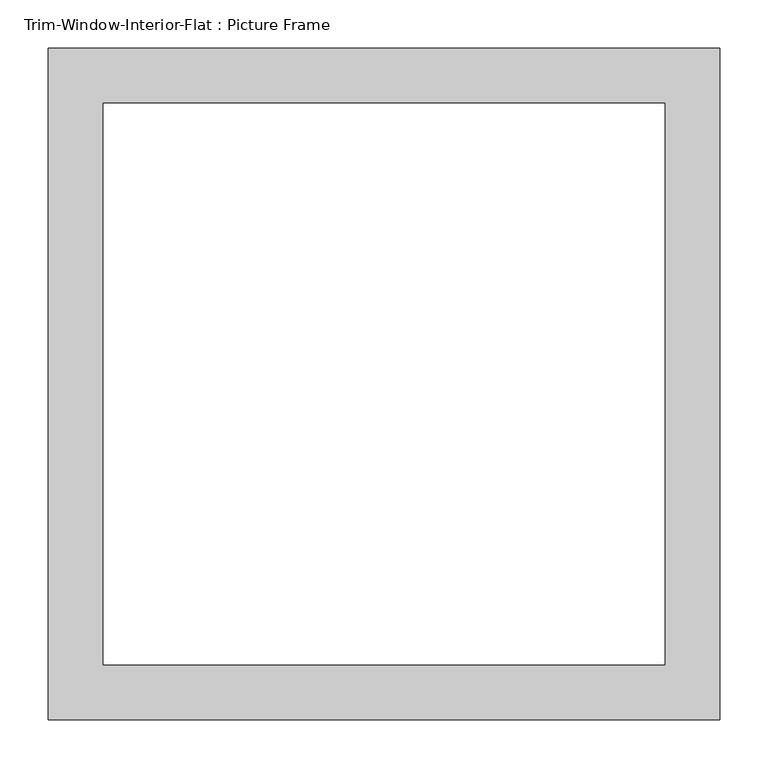
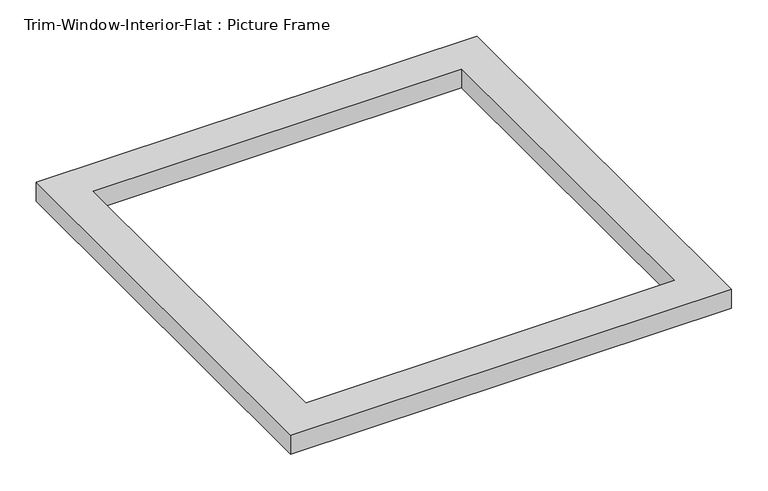
"""IFC4 building model written with IfcOpenShell, lengths in millimetres: proxy geometry, Trim-Window-Interior-Flat : Picture Frame."""

from ifc_helpers import new_model, si_unit, origin, origin_with_axes, place, context, project, spatial, polyline, outline, extrude, source, transform, mapped, element, save


def trim_window_interior_flat_picture_frame_3927330c(model_context):
    return source(origin(), model_context, "Body", "SweptSolid", [
        extrude(outline(polyline([(349.25, 44.45), (349.25, -654.05), (-349.25, -654.05), (-349.25, 44.45), (349.25, 44.45)]), holes=[polyline([(292.1, -12.7), (-292.1, -12.7), (-292.1, -596.9), (292.1, -596.9), (292.1, -12.7)])]), origin_with_axes(), (0.0, 0.0, 1.0), 31.75),
    ])


if __name__ == "__main__":
    model = new_model("IFC4")
    model_context = context("Model", 3, world=origin())
    ifc_project = project(units=[si_unit("LENGTHUNIT", "METRE", prefix="MILLI")], contexts=[model_context])
    site = spatial("IfcSite", under=ifc_project)
    building = spatial("IfcBuilding", under=site)
    placement = place(None, origin())
    trim_window_interior_flat_picture_frame_shape = trim_window_interior_flat_picture_frame_3927330c(model_context)
    element("IfcBuildingElementProxy", 1, Name="Trim-Window-Interior-Flat : Picture Frame", ObjectType="Trim-Window-Interior-Flat : Picture Frame", at=placement, inside=building, context=model_context, shape_type="MappedRepresentation", body=[
        mapped(trim_window_interior_flat_picture_frame_shape, transform((0.0, 0.0, 0.0), x_axis=(1.0, 0.0, 0.0), y_axis=(0.0, 1.0, 0.0), z_axis=(0.0, 0.0, 1.0))),
    ])
    save(model, "model.ifc")

# Revit data of these elements
# Type "Trim-Window-Interior-Flat : Picture Frame"
#   Trim Thickness_Picture Frame = 0' - 1 1/4"
#   Trim Width = 0' - 2 1/4"
#   Trim Thickness_with Sill = 0' - 0 3/4"
#   Sill Thickness = 0' - 1 1/4"
#   Opening Width [instance default] = 2' - 0"
#   Opening Height [instance default] = 3' - 0"
#   Default Elevation = 4' - 0"
#   Sill = no
#   Picture Frame = yes
#   Trim Material [instance default] = none
# Element 1 (IfcBuildingElementProxy, "Trim-Window-Interior-Flat : Picture Frame")
#   Opening Height = 2' - 0"
#   Trim Material = Wood - Stained
#   Materials on its faces: "Wood - Stained"
# Materials
#   "Wood - Stained": class "Wood", colour RGB 224 178 126, transparency 0, Cost = 0
